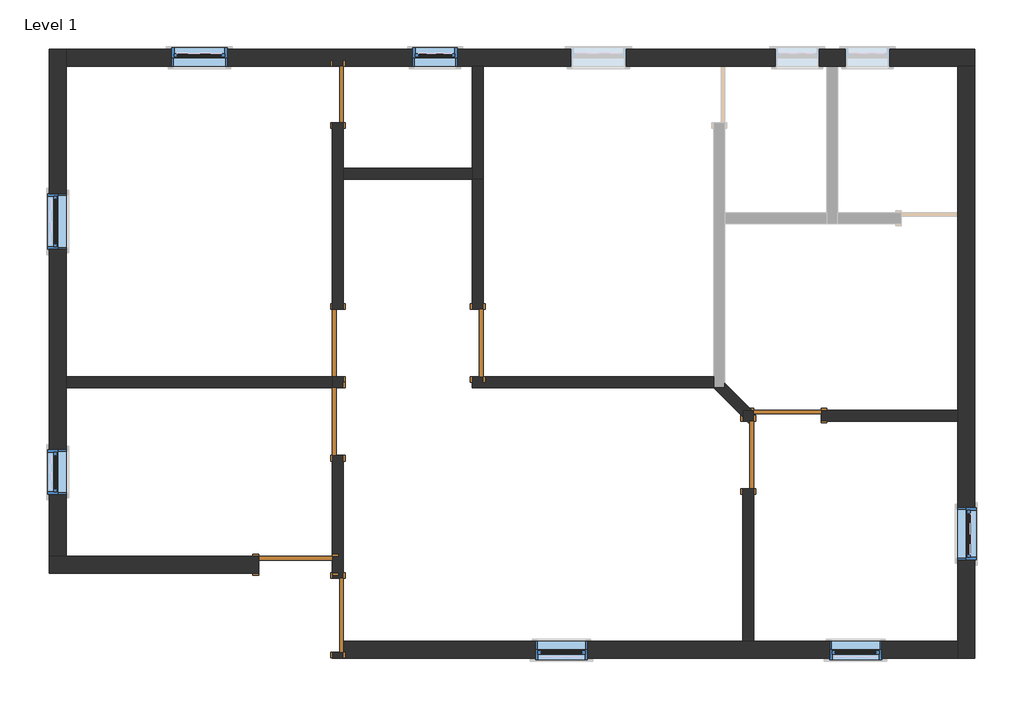
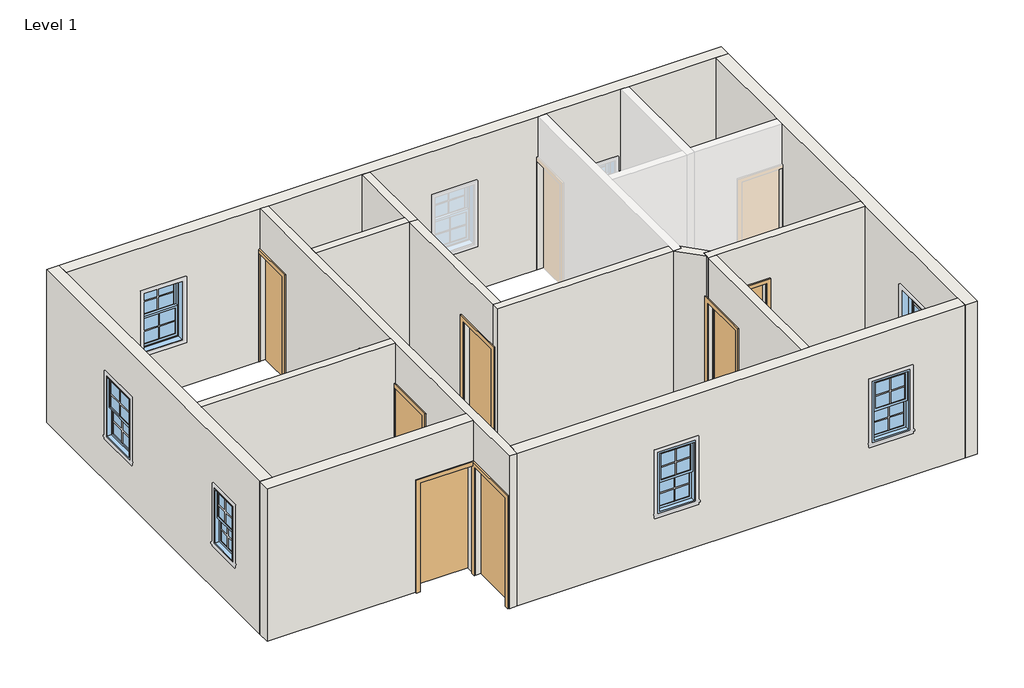
# One storey, part 1 of 2: 14 walls, 8 doors, 7 windows.
"""IFC4 building model written with IfcOpenShell, lengths in millimetres."""

from ifc_helpers import new_model, si_unit, frame, origin, origin_with_axes, place, context, project, spatial, polyline, outline, extrude, faceted_brep, transform, mapped, element, save
from components import m_single_flush_0762_x_2134mm_8c18b9de, m_single_flush_0915_x_2134mm_138fd904, m_single_flush_0915_x_2134mm_f3d7f739, m_single_flush_1000_x_2100_mm_10f5ba11, m_single_flush_1000_x_2100_mm_e4293d47, m_window_double_hung_600_x_1100mm_c7e90a65, m_window_double_hung_600_x_750mm_49d140ec, m_window_double_hung_700_x_1200mm_3a464380, m_window_double_hung_750_x_1200mm_abb80fbd

model = new_model("IFC4")

# Units and contexts
model_context = context("Model", 3, world=origin())
ifc_project = project(units=[si_unit("LENGTHUNIT", "METRE", prefix="MILLI")], contexts=[model_context])

# Site, building, storey
site = spatial("IfcSite", under=ifc_project)
building = spatial("IfcBuilding", under=site)
storey = spatial("IfcBuildingStorey", under=building, Name="Level 1", Elevation=0.0)

# Doors
placement = place(None, origin())
m_single_flush_0762_x_2134mm_shape = m_single_flush_0762_x_2134mm_8c18b9de(model_context)
element("IfcDoor", 1, ObjectType="M_Single-Flush : 0762 x 2134mm", at=placement, inside=storey, context=model_context, shape_type="MappedRepresentation", body=[
    mapped(m_single_flush_0762_x_2134mm_shape, transform((9335.6337578, -14024.8303365, 0.0), x_axis=(0.0, 1.0, 0.0), y_axis=(-1.0, 0.0, 0.0), z_axis=(0.0, 0.0, 1.0))),
])
m_single_flush_0915_x_2134mm_shape = m_single_flush_0915_x_2134mm_138fd904(model_context)
element("IfcDoor", 2, ObjectType="M_Single-Flush : 0915 x 2134mm", at=placement, inside=storey, context=model_context, shape_type="MappedRepresentation", body=[
    mapped(m_single_flush_0915_x_2134mm_shape, transform((9335.6337578, -18451.3303365, 0.0), x_axis=(0.0, 1.0, 0.0), y_axis=(-1.0, 0.0, 0.0), z_axis=(0.0, 0.0, 1.0))),
])
element("IfcDoor", 3, ObjectType="M_Single-Flush : 0915 x 2134mm", at=placement, inside=storey, context=model_context, shape_type="MappedRepresentation", body=[
    mapped(m_single_flush_0915_x_2134mm_shape, transform((11225.6337578, -17386.3303365, 0.0), x_axis=(0.0, -1.0, 0.0), y_axis=(1.0, 0.0, 0.0), z_axis=(0.0, 0.0, 1.0))),
])
element("IfcDoor", 4, ObjectType="M_Single-Flush : 0915 x 2134mm", at=placement, inside=storey, context=model_context, shape_type="MappedRepresentation", body=[
    mapped(m_single_flush_0915_x_2134mm_shape, transform((14885.6337578, -18901.3303365, 0.0), x_axis=(0.0, -1.0, 0.0), y_axis=(1.0, 0.0, 0.0), z_axis=(0.0, 0.0, 1.0))),
])
m_single_flush_0915_x_2134mm_2_shape = m_single_flush_0915_x_2134mm_f3d7f739(model_context)
element("IfcDoor", 5, ObjectType="M_Single-Flush : 0915 x 2134mm", at=placement, inside=storey, context=model_context, shape_type="MappedRepresentation", body=[
    mapped(m_single_flush_0915_x_2134mm_2_shape, transform((9335.6337578, -17386.3303365, 0.0), x_axis=(0.0, -1.0, 0.0), y_axis=(1.0, 0.0, 0.0), z_axis=(0.0, 0.0, 1.0))),
])
element("IfcDoor", 6, ObjectType="M_Single-Flush : 0915 x 2134mm", at=placement, inside=storey, context=model_context, shape_type="MappedRepresentation", body=[
    mapped(m_single_flush_0915_x_2134mm_2_shape, transform((15418.1337578, -18368.8303365, 0.0), x_axis=(-1.0, 0.0, 0.0), y_axis=(0.0, -1.0, 0.0), z_axis=(0.0, 0.0, 1.0))),
])
m_single_flush_1000_x_2100_mm_shape = m_single_flush_1000_x_2100_mm_10f5ba11(model_context)
element("IfcDoor", 7, ObjectType="M_Single-Flush : 1000 X 2100 mm", at=placement, inside=storey, context=model_context, shape_type="MappedRepresentation", body=[
    mapped(m_single_flush_1000_x_2100_mm_shape, transform((8760.6337578, -20388.8303365, 0.0), x_axis=(1.0, 0.0, 0.0), y_axis=(0.0, 1.0, 0.0), z_axis=(0.0, 0.0, 1.0))),
])
m_single_flush_1000_x_2100_mm_2_shape = m_single_flush_1000_x_2100_mm_e4293d47(model_context)
element("IfcDoor", 8, ObjectType="M_Single-Flush : 1000 X 2100 mm", at=placement, inside=storey, context=model_context, shape_type="MappedRepresentation", body=[
    mapped(m_single_flush_1000_x_2100_mm_2_shape, transform((9335.6337578, -21068.8955588, 0.0), x_axis=(0.0, -1.0, 0.0), y_axis=(1.0, 0.0, 0.0), z_axis=(0.0, 0.0, 1.0))),
])

# Walls
element("IfcWall", 9, ObjectType="Exterior-230mm", at=placement, inside=storey, context=model_context, shape_type="Brep", body=[
    faceted_brep([(5430.6337578, -20273.8303365, 3000.0), (5660.6337578, -20273.8303365, 3000.0), (9260.6337578, -20273.8303365, 3000.0), (9260.6337578, -20273.8303365, 2134.0), (8260.6337578, -20273.8303365, 2134.0), (8260.6337578, -20273.8303365, 0.0), (5660.6337578, -20273.8303365, 0.0), (5430.6337578, -20273.8303365, 0.0), (9260.6337578, -20503.8303365, 3000.0), (5430.6337578, -20503.8303365, 3000.0), (5430.6337578, -20503.8303365, 0.0), (8260.6337578, -20503.8303365, 0.0), (8260.6337578, -20503.8303365, 2134.0), (9260.6337578, -20503.8303365, 2134.0)], [[[0, 1, 2, 3, 4, 5, 6, 7]], [[8, 9, 10, 11, 12, 13]], [[10, 7, 6, 5, 11]], [[2, 1, 0, 9, 8]], [[0, 7, 10, 9]], [[2, 8, 13, 3]], [[12, 4, 3, 13]], [[4, 12, 11, 5]]]),
])
element("IfcWall", 10, ObjectType="Exterior-230mm", at=placement, inside=storey, context=model_context, shape_type="Brep", body=[
    faceted_brep([(5660.6337578, -20273.8303365, 0.0), (5660.6337578, -17993.8303365, 0.0), (5660.6337578, -17843.8303365, 0.0), (5660.6337578, -13643.8303365, 0.0), (5660.6337578, -13413.8303365, 0.0), (5660.6337578, -13413.8303365, 3000.0), (5660.6337578, -13643.8303365, 3000.0), (5660.6337578, -17843.8303365, 3000.0), (5660.6337578, -17993.8303365, 3000.0), (5660.6337578, -20273.8303365, 3000.0), (5660.6337578, -19433.8303365, 2014.4), (5660.6337578, -18833.8303365, 2014.4), (5660.6337578, -18833.8303365, 914.4), (5660.6337578, -19433.8303365, 914.4), (5660.6337578, -16118.8303365, 2114.4), (5660.6337578, -15368.8303365, 2114.4), (5660.6337578, -15368.8303365, 914.4), (5660.6337578, -16118.8303365, 914.4), (5430.6337578, -20273.8303365, 0.0), (5430.6337578, -20273.8303365, 3000.0), (5430.6337578, -13413.8303365, 3000.0), (5430.6337578, -13413.8303365, 0.0), (5430.6337578, -19433.8303365, 2014.4), (5430.6337578, -19433.8303365, 914.4), (5430.6337578, -18833.8303365, 914.4), (5430.6337578, -18833.8303365, 2014.4), (5430.6337578, -16118.8303365, 2114.4), (5430.6337578, -16118.8303365, 914.4), (5430.6337578, -15368.8303365, 914.4), (5430.6337578, -15368.8303365, 2114.4)], [[[0, 1, 2, 3, 4, 5, 6, 7, 8, 9], [10, 11, 12, 13], [14, 15, 16, 17]], [[18, 19, 20, 21], [22, 23, 24, 25], [26, 27, 28, 29]], [[4, 3, 2, 1, 0, 18, 21]], [[9, 8, 7, 6, 5, 20, 19]], [[0, 9, 19, 18]], [[5, 4, 21, 20]], [[23, 22, 10, 13]], [[24, 23, 13, 12]], [[25, 24, 12, 11]], [[22, 25, 11, 10]], [[27, 26, 14, 17]], [[28, 27, 17, 16]], [[29, 28, 16, 15]], [[26, 29, 15, 14]]]),
])
element("IfcWall", 11, ObjectType="Exterior-230mm", at=placement, inside=storey, context=model_context, shape_type="Brep", body=[
    faceted_brep([(5660.6337578, -13643.8303365, 0.0), (11150.6337578, -13643.8303365, 0.0), (11300.6337578, -13643.8303365, 0.0), (15950.6337578, -13643.8303365, 0.0), (16100.6337578, -13643.8303365, 0.0), (17720.6337578, -13643.8303365, 0.0), (17950.6337578, -13643.8303365, 0.0), (17950.6337578, -13643.8303365, 3000.0), (17720.6337578, -13643.8303365, 3000.0), (16100.6337578, -13643.8303365, 3000.0), (15950.6337578, -13643.8303365, 3000.0), (14570.6337578, -13643.8303365, 3000.0), (14420.6337578, -13643.8303365, 3000.0), (11300.6337578, -13643.8303365, 3000.0), (11150.6337578, -13643.8303365, 3000.0), (9410.6337578, -13643.8303365, 3000.0), (9260.6337578, -13643.8303365, 3000.0), (5660.6337578, -13643.8303365, 3000.0), (7085.6337578, -13643.8303365, 2114.4), (7835.6337578, -13643.8303365, 2114.4), (7835.6337578, -13643.8303365, 914.4), (7085.6337578, -13643.8303365, 914.4), (12485.6337578, -13643.8303365, 2114.4), (13235.6337578, -13643.8303365, 2114.4), (13235.6337578, -13643.8303365, 914.4), (12485.6337578, -13643.8303365, 914.4), (10350.6337578, -13643.8303365, 1664.4), (10950.6337578, -13643.8303365, 1664.4), (10950.6337578, -13643.8303365, 914.4), (10350.6337578, -13643.8303365, 914.4), (15250.6337578, -13643.8303365, 1664.4), (15850.6337578, -13643.8303365, 1664.4), (15850.6337578, -13643.8303365, 914.4), (15250.6337578, -13643.8303365, 914.4), (16200.6337578, -13643.8303365, 1664.4), (16800.6337578, -13643.8303365, 1664.4), (16800.6337578, -13643.8303365, 914.4), (16200.6337578, -13643.8303365, 914.4), (5660.6337578, -13413.8303365, 0.0), (5660.6337578, -13413.8303365, 3000.0), (17950.6337578, -13413.8303365, 3000.0), (17950.6337578, -13413.8303365, 0.0), (7085.6337578, -13413.8303365, 2114.4), (7085.6337578, -13413.8303365, 914.4), (7835.6337578, -13413.8303365, 914.4), (7835.6337578, -13413.8303365, 2114.4), (12485.6337578, -13413.8303365, 2114.4), (12485.6337578, -13413.8303365, 914.4), (13235.6337578, -13413.8303365, 914.4), (13235.6337578, -13413.8303365, 2114.4), (10350.6337578, -13413.8303365, 1664.4), (10350.6337578, -13413.8303365, 914.4), (10950.6337578, -13413.8303365, 914.4), (10950.6337578, -13413.8303365, 1664.4), (15250.6337578, -13413.8303365, 1664.4), (15250.6337578, -13413.8303365, 914.4), (15850.6337578, -13413.8303365, 914.4), (15850.6337578, -13413.8303365, 1664.4), (16200.6337578, -13413.8303365, 1664.4), (16200.6337578, -13413.8303365, 914.4), (16800.6337578, -13413.8303365, 914.4), (16800.6337578, -13413.8303365, 1664.4)], [[[0, 1, 2, 3, 4, 5, 6, 7, 8, 9, 10, 11, 12, 13, 14, 15, 16, 17], [18, 19, 20, 21], [22, 23, 24, 25], [26, 27, 28, 29], [30, 31, 32, 33], [34, 35, 36, 37]], [[38, 39, 40, 41], [42, 43, 44, 45], [46, 47, 48, 49], [50, 51, 52, 53], [54, 55, 56, 57], [58, 59, 60, 61]], [[6, 5, 4, 3, 2, 1, 0, 38, 41]], [[17, 16, 15, 14, 13, 12, 11, 10, 9, 8, 7, 40, 39]], [[0, 17, 39, 38]], [[7, 6, 41, 40]], [[43, 42, 18, 21]], [[44, 43, 21, 20]], [[45, 44, 20, 19]], [[42, 45, 19, 18]], [[47, 46, 22, 25]], [[48, 47, 25, 24]], [[49, 48, 24, 23]], [[46, 49, 23, 22]], [[51, 50, 26, 29]], [[52, 51, 29, 28]], [[53, 52, 28, 27]], [[50, 53, 27, 26]], [[55, 54, 30, 33]], [[56, 55, 33, 32]], [[57, 56, 32, 31]], [[54, 57, 31, 30]], [[59, 58, 34, 37]], [[60, 59, 37, 36]], [[61, 60, 36, 35]], [[58, 61, 35, 34]]]),
])
element("IfcWall", 12, ObjectType="Exterior-230mm", at=placement, inside=storey, context=model_context, shape_type="Brep", body=[
    faceted_brep([(17720.6337578, -13643.8303365, 0.0), (17720.6337578, -18293.8303365, 0.0), (17720.6337578, -18443.8303365, 0.0), (17720.6337578, -21423.8303365, 0.0), (17720.6337578, -21653.8303365, 0.0), (17720.6337578, -21653.8303365, 3000.0), (17720.6337578, -21423.8303365, 3000.0), (17720.6337578, -18443.8303365, 3000.0), (17720.6337578, -18293.8303365, 3000.0), (17720.6337578, -15773.8303365, 3000.0), (17720.6337578, -15623.8303365, 3000.0), (17720.6337578, -13643.8303365, 3000.0), (17720.6337578, -19618.8303365, 2114.4), (17720.6337578, -20318.8303365, 2114.4), (17720.6337578, -20318.8303365, 914.4), (17720.6337578, -19618.8303365, 914.4), (17950.6337578, -13643.8303365, 0.0), (17950.6337578, -13643.8303365, 3000.0), (17950.6337578, -21653.8303365, 3000.0), (17950.6337578, -21653.8303365, 0.0), (17950.6337578, -19618.8303365, 2114.4), (17950.6337578, -19618.8303365, 914.4), (17950.6337578, -20318.8303365, 914.4), (17950.6337578, -20318.8303365, 2114.4)], [[[0, 1, 2, 3, 4, 5, 6, 7, 8, 9, 10, 11], [12, 13, 14, 15]], [[16, 17, 18, 19], [20, 21, 22, 23]], [[4, 3, 2, 1, 0, 16, 19]], [[11, 10, 9, 8, 7, 6, 5, 18, 17]], [[0, 11, 17, 16]], [[5, 4, 19, 18]], [[21, 20, 12, 15]], [[22, 21, 15, 14]], [[23, 22, 14, 13]], [[20, 23, 13, 12]]]),
])
element("IfcWall", 13, ObjectType="Exterior-230mm", at=placement, inside=storey, context=model_context, shape_type="Brep", body=[
    faceted_brep([(17720.6337578, -21423.8303365, 0.0), (14960.6337578, -21423.8303365, 0.0), (14810.6337578, -21423.8303365, 0.0), (9410.6337578, -21423.8303365, 0.0), (9410.6337578, -21423.8303365, 3000.0), (14810.6337578, -21423.8303365, 3000.0), (14960.6337578, -21423.8303365, 3000.0), (17720.6337578, -21423.8303365, 3000.0), (12710.6337578, -21423.8303365, 2114.4), (12010.6337578, -21423.8303365, 2114.4), (12010.6337578, -21423.8303365, 914.4), (12710.6337578, -21423.8303365, 914.4), (16690.6337578, -21423.8303365, 2114.4), (15990.6337578, -21423.8303365, 2114.4), (15990.6337578, -21423.8303365, 914.4), (16690.6337578, -21423.8303365, 914.4), (17720.6337578, -21653.8303365, 0.0), (17720.6337578, -21653.8303365, 3000.0), (9410.6337578, -21653.8303365, 3000.0), (9410.6337578, -21653.8303365, 0.0), (12710.6337578, -21653.8303365, 2114.4), (12710.6337578, -21653.8303365, 914.4), (12010.6337578, -21653.8303365, 914.4), (12010.6337578, -21653.8303365, 2114.4), (16690.6337578, -21653.8303365, 2114.4), (16690.6337578, -21653.8303365, 914.4), (15990.6337578, -21653.8303365, 914.4), (15990.6337578, -21653.8303365, 2114.4), (9410.6337578, -21568.8955588, 0.0)], [[[0, 1, 2, 3, 4, 5, 6, 7], [8, 9, 10, 11], [12, 13, 14, 15]], [[16, 17, 18, 19], [20, 21, 22, 23], [24, 25, 26, 27]], [[3, 2, 1, 0, 16, 19, 28]], [[7, 6, 5, 4, 18, 17]], [[0, 7, 17, 16]], [[4, 3, 28, 19, 18]], [[21, 20, 8, 11]], [[22, 21, 11, 10]], [[23, 22, 10, 9]], [[20, 23, 9, 8]], [[25, 24, 12, 15]], [[26, 25, 15, 14]], [[27, 26, 14, 13]], [[24, 27, 13, 12]]]),
])
element("IfcWall", 14, ObjectType="Interior-150mm", at=placement, inside=storey, context=model_context, shape_type="Brep", body=[
    faceted_brep([(5660.6337578, -17993.8303365, 0.0), (9260.6337578, -17993.8303365, 0.0), (9260.6337578, -17993.8303365, 2134.0), (9260.6337578, -17993.8303365, 3000.0), (5660.6337578, -17993.8303365, 3000.0), (5660.6337578, -17843.8303365, 0.0), (5660.6337578, -17843.8303365, 3000.0), (9260.6337578, -17843.8303365, 3000.0), (9260.6337578, -17843.8303365, 2134.0), (9260.6337578, -17843.8303365, 0.0)], [[[0, 1, 2, 3, 4]], [[5, 6, 7, 8, 9]], [[1, 0, 5, 9]], [[4, 3, 7, 6]], [[0, 4, 6, 5]], [[3, 2, 1, 9, 8, 7]]]),
])
element("IfcWall", 15, ObjectType="Interior-150mm", at=placement, inside=storey, context=model_context, shape_type="Brep", body=[
    faceted_brep([(9260.6337578, -21568.8955588, 2134.0), (9260.6337578, -21568.8955588, 0.0), (9260.6337578, -21653.8303365, 0.0), (9260.6337578, -21653.8303365, 3000.0), (9260.6337578, -20503.8303365, 3000.0), (9260.6337578, -20273.8303365, 3000.0), (9260.6337578, -17993.8303365, 3000.0), (9260.6337578, -17843.8303365, 3000.0), (9260.6337578, -13643.8303365, 3000.0), (9260.6337578, -13643.8303365, 2134.0), (9260.6337578, -14405.8303365, 2134.0), (9260.6337578, -14405.8303365, 0.0), (9260.6337578, -16928.8303365, 0.0), (9260.6337578, -16928.8303365, 2134.0), (9260.6337578, -17843.8303365, 2134.0), (9260.6337578, -17843.8303365, 0.0), (9260.6337578, -17993.8303365, 0.0), (9260.6337578, -17993.8303365, 2134.0), (9260.6337578, -18908.8303365, 2134.0), (9260.6337578, -18908.8303365, 0.0), (9260.6337578, -20568.8955588, 0.0), (9260.6337578, -20568.8955588, 2134.0), (9410.6337578, -21653.8303365, 0.0), (9410.6337578, -21568.8955588, 0.0), (9410.6337578, -21568.8955588, 2134.0), (9410.6337578, -20568.8955588, 2134.0), (9410.6337578, -20568.8955588, 0.0), (9410.6337578, -18908.8303365, 0.0), (9410.6337578, -18908.8303365, 2134.0), (9410.6337578, -17993.8303365, 2134.0), (9410.6337578, -17993.8303365, 0.0), (9410.6337578, -17843.8303365, 0.0), (9410.6337578, -17843.8303365, 2134.0), (9410.6337578, -16928.8303365, 2134.0), (9410.6337578, -16928.8303365, 0.0), (9410.6337578, -15173.8303365, 0.0), (9410.6337578, -15023.8303365, 0.0), (9410.6337578, -14405.8303365, 0.0), (9410.6337578, -14405.8303365, 2134.0), (9410.6337578, -13643.8303365, 2134.0), (9410.6337578, -13643.8303365, 3000.0), (9410.6337578, -15023.8303365, 3000.0), (9410.6337578, -15173.8303365, 3000.0), (9410.6337578, -21423.8303365, 3000.0), (9410.6337578, -21653.8303365, 3000.0)], [[[0, 1, 2, 3, 4, 5, 6, 7, 8, 9, 10, 11, 12, 13, 14, 15, 16, 17, 18, 19, 20, 21]], [[22, 23, 24, 25, 26, 27, 28, 29, 30, 31, 32, 33, 34, 35, 36, 37, 38, 39, 40, 41, 42, 43, 44]], [[30, 16, 15, 31]], [[34, 12, 11, 37, 36, 35]], [[20, 19, 27, 26]], [[2, 1, 23, 22]], [[8, 7, 6, 5, 4, 3, 44, 43, 42, 41, 40]], [[8, 40, 39, 9]], [[3, 2, 22, 44]], [[17, 16, 30, 29]], [[18, 17, 29, 28]], [[19, 18, 28, 27]], [[32, 31, 15, 14]], [[33, 32, 14, 13]], [[34, 33, 13, 12]], [[38, 10, 9, 39]], [[10, 38, 37, 11]], [[24, 23, 1, 0]], [[25, 24, 0, 21]], [[26, 25, 21, 20]]]),
])
element("IfcWall", 16, ObjectType="Interior-150mm", at=placement, inside=storey, context=model_context, shape_type="Brep", body=[
    faceted_brep([(11150.6337578, -13643.8303365, 0.0), (11150.6337578, -15023.8303365, 0.0), (11150.6337578, -15173.8303365, 0.0), (11150.6337578, -15173.8303365, 3000.0), (11150.6337578, -15023.8303365, 3000.0), (11150.6337578, -13643.8303365, 3000.0), (11300.6337578, -13643.8303365, 0.0), (11300.6337578, -13643.8303365, 3000.0), (11300.6337578, -15173.8303365, 3000.0), (11300.6337578, -15173.8303365, 0.0)], [[[0, 1, 2, 3, 4, 5]], [[6, 7, 8, 9]], [[2, 1, 0, 6, 9]], [[5, 4, 3, 8, 7]], [[0, 5, 7, 6]], [[3, 2, 9, 8]]]),
])
element("IfcWall", 17, ObjectType="Interior-150mm", at=placement, inside=storey, context=model_context, shape_type="SweptSolid", body=[
    extrude(outline(polyline([(9410.6337578, -15023.8303365), (11150.6337578, -15023.8303365), (11150.6337578, -15173.8303365), (9410.6337578, -15173.8303365), (9410.6337578, -15023.8303365)])), origin_with_axes(), (0.0, 0.0, 1.0), 3000.0),
])
element("IfcWall", 18, ObjectType="Interior-150mm", at=placement, inside=storey, context=model_context, shape_type="Brep", body=[
    faceted_brep([(14420.6337578, -17843.8303365, 0.0), (11150.6337578, -17843.8303365, 0.0), (11150.6337578, -17843.8303365, 2134.0), (11150.6337578, -17843.8303365, 3000.0), (11300.6337578, -17843.8303365, 3000.0), (14420.6337578, -17843.8303365, 3000.0), (14420.6337578, -17993.8303365, 0.0), (14420.6337578, -17993.8303365, 3000.0), (11150.6337578, -17993.8303365, 3000.0), (11150.6337578, -17993.8303365, 0.0)], [[[0, 1, 2, 3, 4, 5]], [[6, 7, 8, 9]], [[1, 0, 6, 9]], [[5, 4, 3, 8, 7]], [[3, 2, 1, 9, 8]], [[0, 5, 7, 6]]]),
])
element("IfcWall", 19, ObjectType="Interior-150mm", at=placement, inside=storey, context=model_context, shape_type="SweptSolid", body=[
    extrude(outline(polyline([(-17843.8303365, 3000.0), (-15173.8303365, 3000.0), (-15173.8303365, 0.0), (-16928.8303365, 0.0), (-16928.8303365, 2134.0), (-17843.8303365, 2134.0), (-17843.8303365, 3000.0)])), frame((11150.6337578, 0.0, 0.0), z_axis=(1.0, 0.0, 0.0), x_axis=(0.0, 1.0, 0.0)), (0.0, 0.0, 1.0), 150.0),
])
element("IfcWall", 20, ObjectType="Interior-150mm", at=placement, inside=storey, context=model_context, shape_type="Brep", body=[
    faceted_brep([(14960.6337578, -18293.8303365, 2134.0), (14960.6337578, -18293.8303365, 0.0), (14932.7657921, -18293.8303365, 0.0), (14810.6337578, -18293.8303365, 0.0), (14810.6337578, -18293.8303365, 3000.0), (14932.7657921, -18293.8303365, 3000.0), (17720.6337578, -18293.8303365, 3000.0), (17720.6337578, -18293.8303365, 0.0), (15875.6337578, -18293.8303365, 0.0), (15875.6337578, -18293.8303365, 2134.0), (14810.6337578, -18443.8303365, 0.0), (14960.6337578, -18443.8303365, 0.0), (14960.6337578, -18443.8303365, 2134.0), (15875.6337578, -18443.8303365, 2134.0), (15875.6337578, -18443.8303365, 0.0), (17720.6337578, -18443.8303365, 0.0), (17720.6337578, -18443.8303365, 3000.0), (14960.6337578, -18443.8303365, 3000.0), (14810.6337578, -18443.8303365, 3000.0), (14810.6337578, -18443.8303365, 2134.0), (14810.6337578, -18383.8303365, 0.0), (14810.6337578, -18383.8303365, 3000.0)], [[[0, 1, 2, 3, 4, 5, 6, 7, 8, 9]], [[10, 11, 12, 13, 14, 15, 16, 17, 18, 19]], [[8, 7, 15, 14]], [[3, 2, 1, 11, 10, 20]], [[6, 5, 4, 21, 18, 17, 16]], [[7, 6, 16, 15]], [[4, 3, 20, 10, 19, 18, 21]], [[12, 11, 1, 0]], [[13, 12, 0, 9]], [[14, 13, 9, 8]]]),
])
element("IfcWall", 21, ObjectType="Interior-150mm", at=placement, inside=storey, context=model_context, shape_type="SweptSolid", body=[
    extrude(outline(polyline([(-21423.8303365, 3000.0), (-18443.8303365, 3000.0), (-18443.8303365, 2134.0), (-19358.8303365, 2134.0), (-19358.8303365, 0.0), (-21423.8303365, 0.0), (-21423.8303365, 3000.0)])), frame((14810.6337578, 0.0, 0.0), z_axis=(1.0, 0.0, 0.0), x_axis=(0.0, 1.0, 0.0)), (0.0, 0.0, 1.0), 150.0),
])
element("IfcWall", 22, ObjectType="Interior-150mm", at=placement, inside=storey, context=model_context, shape_type="SweptSolid", body=[
    extrude(outline(polyline([(14810.6337578, -18383.8303365), (14420.6337578, -17993.8303365), (14570.6337578, -17993.8303365), (14570.6337578, -17931.6983022), (14932.7657921, -18293.8303365), (14810.6337578, -18293.8303365), (14810.6337578, -18383.8303365)])), origin_with_axes(), (0.0, 0.0, 1.0), 3000.0),
])

# Windows
m_window_double_hung_600_x_1100mm_shape = m_window_double_hung_600_x_1100mm_c7e90a65(model_context)
element("IfcWindow", 23, ObjectType="M_Window-Double-Hung : 600 x 1100mm", at=placement, inside=storey, context=model_context, shape_type="MappedRepresentation", body=[
    mapped(m_window_double_hung_600_x_1100mm_shape, transform((5545.6337578, -19133.8303365, 0.0), x_axis=(0.0, 1.0, 0.0), y_axis=(-1.0, 0.0, 0.0), z_axis=(0.0, 0.0, 1.0))),
])
m_window_double_hung_600_x_750mm_shape = m_window_double_hung_600_x_750mm_49d140ec(model_context)
element("IfcWindow", 24, ObjectType="M_Window-Double-Hung : 600 x 750mm", at=placement, inside=storey, context=model_context, shape_type="MappedRepresentation", body=[
    mapped(m_window_double_hung_600_x_750mm_shape, transform((10650.6337578, -13528.8303365, 0.0), x_axis=(1.0, 0.0, 0.0), y_axis=(0.0, 1.0, 0.0), z_axis=(0.0, 0.0, 1.0))),
])
m_window_double_hung_700_x_1200mm_shape = m_window_double_hung_700_x_1200mm_3a464380(model_context)
element("IfcWindow", 25, ObjectType="M_Window-Double-Hung : 700 x 1200mm", at=placement, inside=storey, context=model_context, shape_type="MappedRepresentation", body=[
    mapped(m_window_double_hung_700_x_1200mm_shape, transform((12360.6337578, -21538.8303365, 0.0), x_axis=(-1.0, 0.0, 0.0), y_axis=(0.0, -1.0, 0.0), z_axis=(0.0, 0.0, 1.0))),
])
element("IfcWindow", 26, ObjectType="M_Window-Double-Hung : 700 x 1200mm", at=placement, inside=storey, context=model_context, shape_type="MappedRepresentation", body=[
    mapped(m_window_double_hung_700_x_1200mm_shape, transform((16340.6337578, -21538.8303365, 0.0), x_axis=(-1.0, 0.0, 0.0), y_axis=(0.0, -1.0, 0.0), z_axis=(0.0, 0.0, 1.0))),
])
element("IfcWindow", 27, ObjectType="M_Window-Double-Hung : 700 x 1200mm", at=placement, inside=storey, context=model_context, shape_type="MappedRepresentation", body=[
    mapped(m_window_double_hung_700_x_1200mm_shape, transform((17835.6337578, -19968.8303365, 0.0), x_axis=(0.0, -1.0, 0.0), y_axis=(1.0, 0.0, 0.0), z_axis=(0.0, 0.0, 1.0))),
])
m_window_double_hung_750_x_1200mm_shape = m_window_double_hung_750_x_1200mm_abb80fbd(model_context)
element("IfcWindow", 28, ObjectType="M_Window-Double-Hung : 750 x 1200mm", at=placement, inside=storey, context=model_context, shape_type="MappedRepresentation", body=[
    mapped(m_window_double_hung_750_x_1200mm_shape, transform((5545.6337578, -15743.8303365, 0.0), x_axis=(0.0, 1.0, 0.0), y_axis=(-1.0, 0.0, 0.0), z_axis=(0.0, 0.0, 1.0))),
])
element("IfcWindow", 29, ObjectType="M_Window-Double-Hung : 750 x 1200mm", at=placement, inside=storey, context=model_context, shape_type="MappedRepresentation", body=[
    mapped(m_window_double_hung_750_x_1200mm_shape, transform((7460.6337578, -13528.8303365, 0.0), x_axis=(1.0, 0.0, 0.0), y_axis=(0.0, 1.0, 0.0), z_axis=(0.0, 0.0, 1.0))),
])

save(model, "model.ifc")

# Revit data of these elements
# Type "M_Single-Flush : 0762 x 2134mm"
#   Type Mark = "26"
#   Construction Type Id = "MDOOR"
#   Analytic Construction = "Metal"
#   Thickness = 0.051 m
#   Thermal Resistance (R) = 0.270117 (m²·K)/W
#   Heat Transfer Coefficient (U) = 3.7021 W/(m²·K)
#   Height = 2.134 m
#   Trim Projection Ext = 0.025 m
#   Trim Projection Int = 0.025 m
#   Trim Width = 0.076 m
#   Width = 0.762 m
#   Define Thermal Properties by = 1
#   Define Thermal Properties by = 1
#   Door Material = Door - Panel
#   Frame Material = Door - Frame
#   Visual Light Transmittance = 0
#   Solar Heat Gain Coefficient = 0
#   Function = (empty or 0)
#   Wall Closure = (empty or 0)
# Type "M_Single-Flush : 0915 x 2134mm"
#   Type Mark = "20"
#   Construction Type Id = "MDOOR"
#   Analytic Construction = "Metal"
#   Thickness = 0.051 m
#   Thermal Resistance (R) = 0.270117 (m²·K)/W
#   Heat Transfer Coefficient (U) = 3.7021 W/(m²·K)
#   Height = 2.134 m
#   Trim Projection Ext = 0.025 m
#   Trim Projection Int = 0.025 m
#   Trim Width = 0.076 m
#   Width = 0.915 m
#   Define Thermal Properties by = 1
#   Define Thermal Properties by = 1
#   Door Material = Door - Panel
#   Frame Material = Door - Frame
#   Visual Light Transmittance = 0
#   Solar Heat Gain Coefficient = 0
#   Function = (empty or 0)
#   Wall Closure = (empty or 0)
# Type "M_Single-Flush : 1000 X 2100 mm"
#   Type Mark = "40"
#   Construction Type Id = "MDOOR"
#   Analytic Construction = "Metal"
#   Thickness = 0.051 m
#   Thermal Resistance (R) = 0.270117 (m²·K)/W
#   Heat Transfer Coefficient (U) = 3.7021 W/(m²·K)
#   Height = 2.134 m
#   Trim Projection Ext = 0.025 m
#   Trim Projection Int = 0.025 m
#   Trim Width = 0.076 m
#   Width = 1 m
#   Define Thermal Properties by = 1
#   Door Material = Door - Panel
#   Frame Material = Door - Frame
#   Visual Light Transmittance = 0
#   Solar Heat Gain Coefficient = 0
#   Function = (empty or 0)
#   Wall Closure = (empty or 0)
# Type "Exterior-230mm"
#   Layers, outside or top first: 0.23 m no material (function 1)
# Type "Interior-150mm"
#   Layers, outside or top first: 0.15 m no material (function 1)
# Type "M_Window-Double-Hung : 600 x 1100mm"
#   Type Mark = "W1"
#   Fire Rating = "0.5h"
#   Construction Type Id = "DG-DR"
#   Assembly Code = "B2020100"
#   Analytic Construction = "Double glazing - domestic"
#   Wall Thickness [instance default] = 0.15 m
#   Window Inset [instance default] = 0 m
#   Visual Light Transmittance = 0.81
#   Thermal Resistance (R) = 0.319569 (m²·K)/W
#   Solar Heat Gain Coefficient = 0.76
#   Muntin Width = 0.4476 m
#   Muntin Height = 0.451575 m
#   Interior Wall Closure [instance default] = 0.0357 m
#   Rough Width = 0.615 m
#   Rough Height = 1.115 m
#   Frame Extension [instance default] = 0.03175 m
#   Exterior Wall Closure [instance default] = 0.0127 m
#   Extension Jamb [instance default] = 0.0357 m
#   Heat Transfer Coefficient (U) = 3.12929 W/(m²·K)
#   Height = 1.1 m
#   Width = 0.6 m
#   Define Thermal Properties by = 1
#   Top Muntin Visibility = yes
#   Indicator Visibility [instance default] = yes
#   Extension Jamb Visibility [instance default] = yes
#   Interior Trim Visibility [instance default] = yes
#   Exterior Trim Visibility [instance default] = yes
#   Define Thermal Properties by = 1
#   Bottom Muntin Visibility = yes
#   Muntin Pattern = M_Muntin Pattern_2x2 : M_Muntin Pattern_2x2
#   Interior Trim Material = Wood - Stained
#   Interior Trim = M_Trim-Window-Interior-Flat : Picture Frame
#   Exterior Trim Material = Clad - White
#   Exterior Trim = M_Trim-Window-Exterior-Flat : with Sill
#   Glass Panel Material = Glass
#   Exterior Frame Material = Clad - White
#   Interior Frame Material = Wood - Stained
#   Wall Closure = (empty or 0)
# Type "M_Window-Double-Hung : 600 x 750mm"
#   Type Mark = "V"
#   Fire Rating = "0.5h"
#   Construction Type Id = "DG-DR"
#   Assembly Code = "B2020100"
#   Analytic Construction = "Double glazing - domestic"
#   Wall Thickness [instance default] = 0.15 m
#   Window Inset [instance default] = 0 m
#   Visual Light Transmittance = 0.81
#   Thermal Resistance (R) = 0.319569 (m²·K)/W
#   Solar Heat Gain Coefficient = 0.76
#   Muntin Width = 0.4476 m
#   Muntin Height = 0.276575 m
#   Interior Wall Closure [instance default] = 0.0357 m
#   Rough Width = 0.615 m
#   Rough Height = 0.765 m
#   Frame Extension [instance default] = 0.03175 m
#   Exterior Wall Closure [instance default] = 0.0127 m
#   Extension Jamb [instance default] = 0.0357 m
#   Heat Transfer Coefficient (U) = 3.12929 W/(m²·K)
#   Height = 0.75 m
#   Width = 0.6 m
#   Top Muntin Visibility = yes
#   Indicator Visibility [instance default] = yes
#   Extension Jamb Visibility [instance default] = yes
#   Interior Trim Visibility [instance default] = yes
#   Exterior Trim Visibility [instance default] = yes
#   Define Thermal Properties by = 1
#   Bottom Muntin Visibility = yes
#   Muntin Pattern = M_Muntin Pattern_2x2 : M_Muntin Pattern_2x2
#   Interior Trim Material = Wood - Stained
#   Interior Trim = M_Trim-Window-Interior-Flat : Picture Frame
#   Exterior Trim Material = Clad - White
#   Exterior Trim = M_Trim-Window-Exterior-Flat : with Sill
#   Glass Panel Material = Glass
#   Exterior Frame Material = Clad - White
#   Interior Frame Material = Wood - Stained
#   Wall Closure = (empty or 0)
# Type "M_Window-Double-Hung : 700 x 1200mm"
#   Type Mark = "W3"
#   Fire Rating = "0.5h"
#   Construction Type Id = "DG-DR"
#   Assembly Code = "B2020100"
#   Analytic Construction = "Double glazing - domestic"
#   Wall Thickness [instance default] = 0.15 m
#   Window Inset [instance default] = 0 m
#   Visual Light Transmittance = 0.81
#   Thermal Resistance (R) = 0.319569 (m²·K)/W
#   Solar Heat Gain Coefficient = 0.76
#   Muntin Width = 0.5476 m
#   Muntin Height = 0.501575 m
#   Interior Wall Closure [instance default] = 0.0357 m
#   Rough Width = 0.715 m
#   Rough Height = 1.215 m
#   Frame Extension [instance default] = 0.03175 m
#   Exterior Wall Closure [instance default] = 0.0127 m
#   Extension Jamb [instance default] = 0.0357 m
#   Heat Transfer Coefficient (U) = 3.12929 W/(m²·K)
#   Height = 1.2 m
#   Width = 0.7 m
#   Define Thermal Properties by = 1
#   Top Muntin Visibility = yes
#   Indicator Visibility [instance default] = yes
#   Extension Jamb Visibility [instance default] = yes
#   Interior Trim Visibility [instance default] = yes
#   Exterior Trim Visibility [instance default] = yes
#   Define Thermal Properties by = 1
#   Bottom Muntin Visibility = yes
#   Muntin Pattern = M_Muntin Pattern_2x2 : M_Muntin Pattern_2x2
#   Interior Trim Material = Wood - Stained
#   Interior Trim = M_Trim-Window-Interior-Flat : Picture Frame
#   Exterior Trim Material = Clad - White
#   Exterior Trim = M_Trim-Window-Exterior-Flat : with Sill
#   Glass Panel Material = Glass
#   Exterior Frame Material = Clad - White
#   Interior Frame Material = Wood - Stained
#   Wall Closure = (empty or 0)
# Type "M_Window-Double-Hung : 750 x 1200mm"
#   Type Mark = "W2"
#   Fire Rating = "0.5h"
#   Construction Type Id = "DG-DR"
#   Assembly Code = "B2020100"
#   Analytic Construction = "Double glazing - domestic"
#   Wall Thickness [instance default] = 0.15 m
#   Window Inset [instance default] = 0 m
#   Visual Light Transmittance = 0.81
#   Thermal Resistance (R) = 0.319569 (m²·K)/W
#   Solar Heat Gain Coefficient = 0.76
#   Muntin Width = 0.5976 m
#   Muntin Height = 0.501575 m
#   Interior Wall Closure [instance default] = 0.0357 m
#   Rough Width = 0.765 m
#   Rough Height = 1.215 m
#   Frame Extension [instance default] = 0.03175 m
#   Exterior Wall Closure [instance default] = 0.0127 m
#   Extension Jamb [instance default] = 0.0357 m
#   Heat Transfer Coefficient (U) = 3.12929 W/(m²·K)
#   Height = 1.2 m
#   Width = 0.75 m
#   Define Thermal Properties by = 1
#   Top Muntin Visibility = yes
#   Indicator Visibility [instance default] = yes
#   Extension Jamb Visibility [instance default] = yes
#   Interior Trim Visibility [instance default] = yes
#   Exterior Trim Visibility [instance default] = yes
#   Define Thermal Properties by = 1
#   Bottom Muntin Visibility = yes
#   Muntin Pattern = M_Muntin Pattern_2x2 : M_Muntin Pattern_2x2
#   Interior Trim Material = Wood - Stained
#   Interior Trim = M_Trim-Window-Interior-Flat : Picture Frame
#   Exterior Trim Material = Clad - White
#   Exterior Trim = M_Trim-Window-Exterior-Flat : with Sill
#   Glass Panel Material = Glass
#   Exterior Frame Material = Clad - White
#   Interior Frame Material = Wood - Stained
#   Wall Closure = (empty or 0)
# Element 1 (IfcDoor, "M_Single-Flush : 0762 x 2134mm")
#   Phase Created = New Construction
#   Materials on its faces: "Door - Frame", "Door - Panel"
# Elements 2, 3, 4, 5, 6 (IfcDoor, "M_Single-Flush : 0915 x 2134mm")
#   Phase Created = New Construction
#   Materials on its faces: "Door - Frame", "Door - Panel"
# Elements 7, 8 (IfcDoor, "M_Single-Flush : 1000 X 2100 mm")
#   Phase Created = New Construction
#   Materials on its faces: "Door - Frame", "Door - Panel"
# Elements 9, 10, 11, 12, 13 (IfcWall, "Exterior-230mm")
#   Top Offset = 0 m
#   Base Offset = 0 m
#   wall height = 3 m
#   Phase Created = New Construction
#   Base Constraint = Level 1
#   Top Constraint = Level 2
#   Materials on its faces: "Default Wall"
# Elements 14, 15, 16, 17, 18, 19, 20, 21, 22 (IfcWall, "Interior-150mm")
#   Top Offset = 0 m
#   Base Offset = 0 m
#   wall height = 3 m
#   Phase Created = New Construction
#   Base Constraint = Level 1
#   Top Constraint = Level 2
#   Materials on its faces: "Default Wall"
# Element 23 (IfcWindow, "M_Window-Double-Hung : 600 x 1100mm")
#   Mark = "1"
#   Window Inset = 0 m
#   Interior Wall Closure = 0.0357 m
#   Frame Extension = 0.03175 m
#   Exterior Wall Closure = 0.0127 m
#   Interior Trim Visibility = yes
#   Indicator Visibility = yes
#   Exterior Trim Visibility = yes
#   Phase Created = New Construction
#   Materials on its faces: "Wood - Stained", "Glass", "Clad - White"
# Element 24 (IfcWindow, "M_Window-Double-Hung : 600 x 750mm")
#   Mark = "11"
#   Window Inset = 0 m
#   Interior Wall Closure = 0.0357 m
#   Frame Extension = 0.03175 m
#   Exterior Wall Closure = 0.0127 m
#   Interior Trim Visibility = yes
#   Indicator Visibility = yes
#   Exterior Trim Visibility = yes
#   Phase Created = New Construction
#   Materials on its faces: "Wood - Stained", "Glass", "Clad - White"
# Element 25 (IfcWindow, "M_Window-Double-Hung : 700 x 1200mm")
#   Mark = "8"
#   Window Inset = 0 m
#   Interior Wall Closure = 0.0357 m
#   Frame Extension = 0.03175 m
#   Exterior Wall Closure = 0.0127 m
#   Interior Trim Visibility = yes
#   Indicator Visibility = yes
#   Exterior Trim Visibility = yes
#   Phase Created = New Construction
#   Materials on its faces: "Wood - Stained", "Glass", "Clad - White"
# Element 26 (IfcWindow, "M_Window-Double-Hung : 700 x 1200mm")
#   Mark = "9"
#   Window Inset = 0 m
#   Interior Wall Closure = 0.0357 m
#   Frame Extension = 0.03175 m
#   Exterior Wall Closure = 0.0127 m
#   Interior Trim Visibility = yes
#   Indicator Visibility = yes
#   Exterior Trim Visibility = yes
#   Phase Created = New Construction
#   Materials on its faces: "Wood - Stained", "Glass", "Clad - White"
# Element 27 (IfcWindow, "M_Window-Double-Hung : 700 x 1200mm")
#   Mark = "10"
#   Window Inset = 0 m
#   Interior Wall Closure = 0.0357 m
#   Frame Extension = 0.03175 m
#   Exterior Wall Closure = 0.0127 m
#   Interior Trim Visibility = yes
#   Indicator Visibility = yes
#   Exterior Trim Visibility = yes
#   Phase Created = New Construction
#   Materials on its faces: "Wood - Stained", "Glass", "Clad - White"
# Element 28 (IfcWindow, "M_Window-Double-Hung : 750 x 1200mm")
#   Mark = "5"
#   Window Inset = 0 m
#   Interior Wall Closure = 0.0357 m
#   Frame Extension = 0.03175 m
#   Exterior Wall Closure = 0.0127 m
#   Interior Trim Visibility = yes
#   Indicator Visibility = yes
#   Exterior Trim Visibility = yes
#   Phase Created = New Construction
#   Materials on its faces: "Wood - Stained", "Glass", "Clad - White"
# Element 29 (IfcWindow, "M_Window-Double-Hung : 750 x 1200mm")
#   Mark = "6"
#   Window Inset = 0 m
#   Interior Wall Closure = 0.0357 m
#   Frame Extension = 0.03175 m
#   Exterior Wall Closure = 0.0127 m
#   Interior Trim Visibility = yes
#   Indicator Visibility = yes
#   Exterior Trim Visibility = yes
#   Phase Created = New Construction
#   Materials on its faces: "Wood - Stained", "Glass", "Clad - White"
# Materials
#   "Door - Panel": class "Wood", colour RGB 210 159 95, transparency 0, Cost = 0
#   "Door - Frame": colour RGB 118 70 51, transparency 0, Cost = 0
#   "Wood - Stained": class "Wood", colour RGB 224 178 126, transparency 0, Cost = 0
#   "Clad - White": class "Wood", colour RGB 242 242 238, transparency 0, Cost = 0
#   "Glass": class "Glass", colour RGB 0 128 192, transparency 0.9, Description = "Soda Lime Glass", Cost = 0
#   "Default Wall": colour RGB 128 128 128, transparency 0, Cost = 0
# Room at (7468.446, -15747.539) mm, phase "New Construction", upper level "Level 1", upper offset 4 m, lower offset 0 m
#   Number = "1"
#   Name = "BEDROOM"
# Room at (10288.466, -14284.507) mm, phase "New Construction", upper level "Level 1", upper offset 4 m, lower offset 0 m
#   Number = "2"
#   Name = "TOILET"
# Room at (13120.302, -15395.134) mm, phase "New Construction", upper level "Level 1", upper offset 4 m, lower offset 0 m
#   Number = "3"
#   Name = "BEDROOM"
# Room at (15338.751, -14528.323) mm, phase "New Construction", upper level "Level 1", upper offset 4 m, lower offset 0 m
#   Number = "4"
#   Name = "TOILET"
# Room at (16925.457, -14735.323) mm, phase "New Construction", upper level "Level 1", upper offset 4 m, lower offset 0 m
#   Number = "5"
#   Name = "TOILET"
# Room at (16138.751, -16996.532) mm, phase "New Construction", upper level "Level 1", upper offset 4 m, lower offset 0 m
#   Number = "6"
#   Name = "DINING"
# Room at (16396.555, -19876.108) mm, phase "New Construction", upper level "Level 1", upper offset 4 m, lower offset 0 m
#   Number = "7"
#   Name = "KITCHEN"
# Room, not placed, phase "New Construction", upper offset 0 m, lower offset 0 m
#   Number = "8"
#   Name = "Room"
# Room at (7468.446, -19025.305) mm, phase "New Construction", upper level "Level 1", upper offset 4 m, lower offset 0 m
#   Number = "9"
#   Name = "OFFICE"
# Room at (12067.923, -19685.116) mm, phase "New Construction", upper level "Level 1", upper offset 4 m, lower offset 0 m
#   Number = "10"
#   Name = "LIVING ROOM"
# Room at (10260.952, -16407.35) mm, phase "New Construction", upper level "Level 1", upper offset 4 m, lower offset 0 m
#   Number = "11"
#   Name = "PASSAGE"
